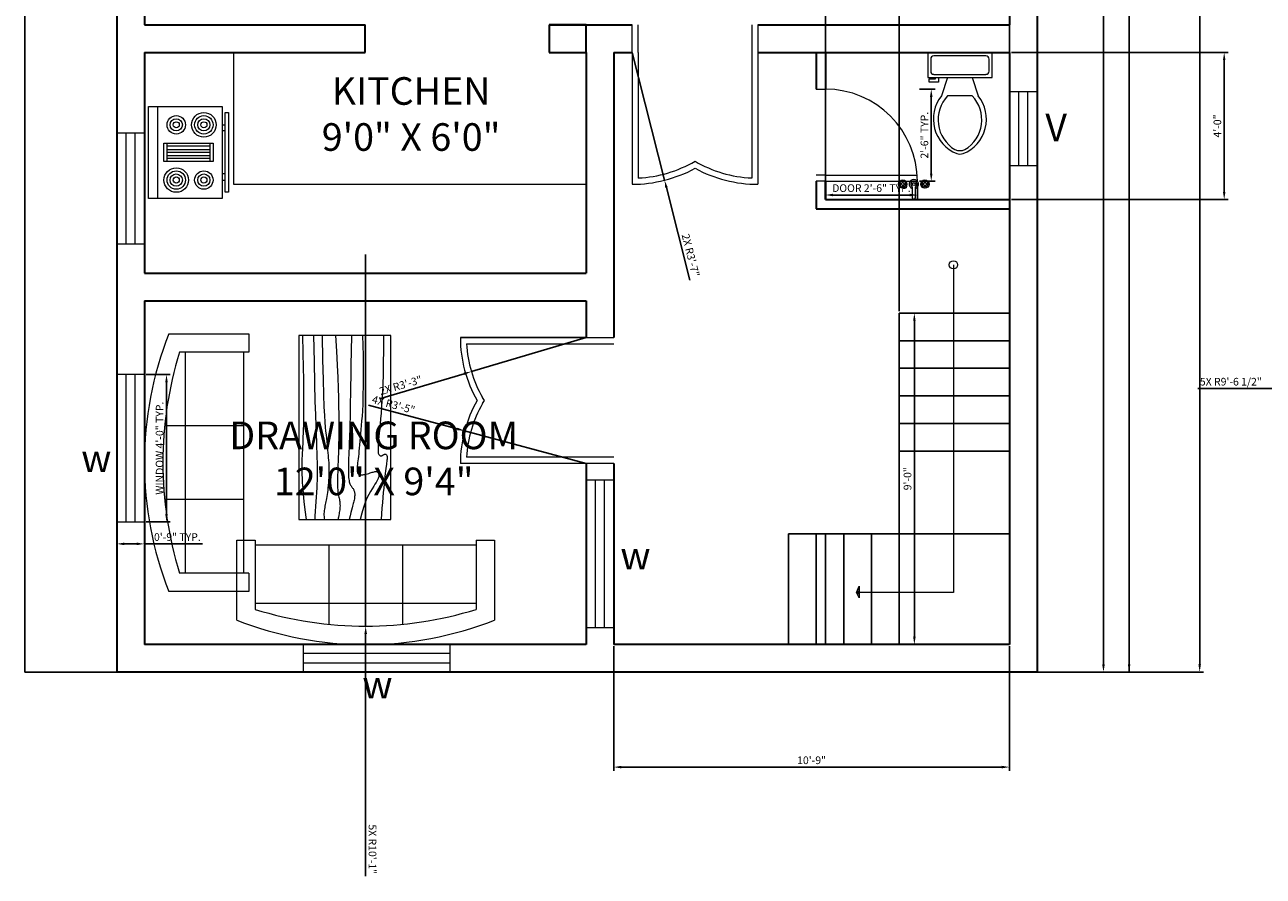
# Model space of a CAD drawing. Units: inches. Extents: x 2009 to 2890, y 2827 to 3504.
# Tile 1 of 6: x 2046 to 2449, y 2827 to 3105. Entities that reach past the tile are written whole.
import ezdxf

# ---------------------------------------------------------------- set-up
doc = ezdxf.new("R2010")
doc.units = ezdxf.units.IN
for name, color, linetype, lineweight in [('A-ANNO-DIMS', 2, 'Continuous', 18), ('A-ANNO-SYMB', 2, 'Continuous', 18), ('A-ANNO-TEXT', 3, 'Continuous', 18), ('A-AREA-IDEN', 7, 'Continuous', 25), ('A-DOOR', 3, 'Continuous', 18), ('A-EQPM', 9, 'Continuous', 18), ('A-FLOR-CASE', 32, 'Continuous', 20), ('A-FLOR-FIXT', 9, 'Continuous', 18), ('A-FLOR-STRS', 7, 'Continuous', 25), ('A-FURN', 8, 'Continuous', 18), ('A-GLAZ', 4, 'Continuous', 18), ('A-WALL', 7, 'Continuous', 35), ('C-PROP', 8, 'Continuous', 25)]:
    doc.layers.add(name, color=color, linetype=linetype, lineweight=lineweight)
doc.styles.get("Standard").update_dxf_attribs({"font": 'arial.ttf'})
doc.dimstyles.new('ISO-25', dxfattribs={"dimtxt": 2.5, "dimasz": 2.5, "dimexe": 1.25, "dimexo": 0.625, "dimtad": 1, "dimdec": 0, "dimlunit": 3, "dimtxsty": 'Standard', "dimcen": 2.5, "dimadec": 0, "dimazin": 0, "dimtfac": 1, "dimtdec": 0, "dimtmove": 0, "dimatfit": 3, "dimfxl": 1, "dimarcsym": 0})

# ---------------------------------------------------------------- blocks, each defined once
blk = doc.blocks.new('Table - Rectangular Woodgrain 60 x 30 in.')
for p, q in [((0, 0), (0, -30)), ((60, 0), (0, 0)), ((60, -30), (60, 0)), ((0, -30), (60, -30))]:
    blk.add_line(p, q)
for points in [[(0, -2.4), (4.8155, -2.418), (9.0302, -2.4688), (12.709, -2.5477), (15.9167, -2.65), (18.7181, -2.7711), (21.1781, -2.9063), (23.3616, -3.0508), (25.3333, -3.2), (27.1477, -3.3495), (28.8172, -3.4958), (30.3437, -3.636), (31.7291, -3.7667), (32.9756, -3.8849), (34.0849, -3.9875), (35.059, -4.0714), (35.9, -4.1334), (36.6114, -4.1711), (37.2041, -4.1854), (37.6906, -4.1779), (38.0833, -4.15), (38.3948, -4.1034), (38.6375, -4.0396), (38.8239, -3.9602), (38.9666, -3.8667), (39.0764, -3.7608), (39.1573, -3.6448), (39.2116, -3.521), (39.2416, -3.3917), (39.2498, -3.2593), (39.2385, -3.1261), (39.21, -2.9944), (39.1666, -2.8667), (39.111, -2.7447), (39.0468, -2.6281), (38.978, -2.5163), (38.9083, -2.4083), (38.8418, -2.3035), (38.7823, -2.201), (38.7337, -2.1001), (38.7, -2), (38.6844, -1.9003), (38.6875, -1.8021), (38.7094, -1.707), (38.75, -1.6167), (38.8094, -1.5326), (38.8875, -1.4563), (38.9844, -1.3893), (39.1, -1.3333), (39.2351, -1.2896), (39.3937, -1.2583), (39.5804, -1.2396), (39.8, -1.2333), (40.057, -1.2396), (40.3562, -1.2583), (40.7023, -1.2896), (41.1, -1.3333), (41.5547, -1.3895), (42.0755, -1.4573), (42.6721, -1.5361), (43.3542, -1.625), (44.1316, -1.7233), (45.014, -1.8302), (46.0114, -1.9449), (47.1333, -2.0667), (48.3862, -2.1947), (49.7625, -2.3281), (51.2513, -2.4663), (52.8416, -2.6083), (54.5226, -2.7535), (56.2833, -2.9011), (58.1127, -3.0501), (60, -3.2)], [(0, -9.2), (6.5759, -9.0858), (11.9385, -9.0365), (16.2527, -9.0418), (19.6833, -9.0917), (22.3952, -9.1759), (24.5531, -9.2844), (26.322, -9.4069), (27.8666, -9.5333), (29.3241, -9.6553), (30.7203, -9.7719), (32.0532, -9.8837), (33.3208, -9.9917), (34.5213, -10.0965), (35.6526, -10.199), (36.7128, -10.2999), (37.7, -10.4), (38.6129, -10.4996), (39.4531, -10.5969), (40.223, -10.6895), (40.925, -10.775), (41.5613, -10.8512), (42.1344, -10.9156), (42.6465, -10.966), (43.1, -11), (43.4976, -11.0158), (43.8437, -11.0136), (44.143, -10.9942), (44.4, -10.9583), (44.6195, -10.9069), (44.8062, -10.8406), (44.9648, -10.7603), (45.1, -10.6667), (45.2155, -10.5598), (45.3114, -10.4365), (45.3871, -10.2929), (45.4416, -10.125), (45.4743, -9.929), (45.4844, -9.7011), (45.4709, -9.4371), (45.4333, -9.1333), (45.3716, -8.7883), (45.2896, -8.4104), (45.1919, -8.0107), (45.0833, -7.6), (44.9685, -7.1893), (44.8521, -6.7896), (44.7388, -6.4117), (44.6333, -6.0667), (44.54, -5.7628), (44.4614, -5.4979), (44.4001, -5.2675), (44.3583, -5.0667), (44.3384, -4.8909), (44.3427, -4.7354), (44.3736, -4.5956), (44.4333, -4.4667), (44.5236, -4.3453), (44.6427, -4.2333), (44.7884, -4.1339), (44.9583, -4.05), (45.1501, -3.9849), (45.3614, -3.9417), (45.59, -3.9234), (45.8333, -3.9333), (46.0915, -3.9749), (46.3734, -4.0531), (46.6906, -4.1736), (47.0542, -4.3417), (47.4756, -4.5629), (47.9661, -4.8427), (48.5372, -5.1866), (49.2, -5.6), (49.9676, -6.0844), (50.8594, -6.625), (51.8965, -7.2031), (53.1, -7.8), (54.491, -8.3969), (56.0906, -8.975), (57.9199, -9.5156), (60, -10)], [(0, -12.8), (5.1847, -12.9322), (9.6213, -13.0323), (13.3963, -13.1059), (16.5958, -13.1583), (19.3063, -13.1952), (21.614, -13.2219), (23.6054, -13.2439), (25.3666, -13.2667), (26.9728, -13.2947), (28.4531, -13.3281), (29.8256, -13.3663), (31.1083, -13.4083), (32.3191, -13.4535), (33.476, -13.501), (34.597, -13.5501), (35.7, -13.6), (36.7984, -13.6497), (37.8875, -13.6979), (38.9578, -13.743), (40, -13.7833), (41.0047, -13.8174), (41.9625, -13.8438), (42.864, -13.8607), (43.7, -13.8667), (44.4631, -13.8604), (45.1552, -13.8417), (45.7801, -13.8104), (46.3416, -13.7667), (46.8439, -13.7104), (47.2906, -13.6417), (47.6858, -13.5604), (48.0333, -13.4667), (48.3375, -13.3608), (48.6042, -13.2448), (48.8396, -13.121), (49.05, -12.9917), (49.2417, -12.8593), (49.4208, -12.7261), (49.5937, -12.5944), (49.7667, -12.4667), (49.9452, -12.3451), (50.1323, -12.2313), (50.3303, -12.1268), (50.5416, -12.0333), (50.7686, -11.9524), (51.0135, -11.8854), (51.2788, -11.8341), (51.5666, -11.8), (51.8785, -11.7843), (52.2116, -11.7865), (52.562, -11.8059), (52.926, -11.8417), (53.2998, -11.8931), (53.6795, -11.9594), (54.0614, -12.0397), (54.4416, -12.1333), (54.8223, -12.2401), (55.2293, -12.3625), (55.6942, -12.5037), (56.2489, -12.6667), (56.9251, -12.8547), (57.7545, -13.0708), (58.7689, -13.3182), (60, -13.6)], [(0, -18), (5.124, -17.7273), (9.6609, -17.5057), (13.6705, -17.3303), (17.2125, -17.1958), (20.3467, -17.0973), (23.1328, -17.0297), (25.6307, -16.9878), (27.9, -16.9667), (29.9928, -16.9617), (31.9302, -16.9703), (33.7254, -16.9907), (35.3917, -17.0208), (36.9423, -17.0588), (38.3906, -17.1026), (39.7499, -17.1503), (41.0333, -17.2), (42.2519, -17.2496), (43.4073, -17.2969), (44.4986, -17.3395), (45.525, -17.375), (46.4858, -17.4012), (47.3802, -17.4156), (48.2074, -17.416), (48.9667, -17.4), (49.6583, -17.3662), (50.2872, -17.3167), (50.8595, -17.2547), (51.3812, -17.1833), (51.8584, -17.1057), (52.2971, -17.025), (52.7034, -16.9443), (53.0833, -16.8667), (53.443, -16.7951), (53.789, -16.7313), (54.128, -16.6768), (54.4666, -16.6334), (54.8115, -16.6024), (55.1693, -16.5854), (55.5465, -16.5841), (55.95, -16.6), (56.3828, -16.6337), (56.8346, -16.6823), (57.2915, -16.7418), (57.7396, -16.8084), (58.165, -16.878), (58.5539, -16.9469), (58.8924, -17.0111), (59.1666, -17.0667), (59.3679, -17.1107), (59.5078, -17.1438), (59.6032, -17.1675), (59.6708, -17.1833), (59.7275, -17.193), (59.7901, -17.1979), (59.8753, -17.1998), (60, -17.2)], [(0, -22.4), (8.0098, -22.2501), (14.4094, -22.1011), (19.4168, -21.9535), (23.25, -21.8083), (26.1269, -21.6663), (28.2656, -21.5281), (29.884, -21.3947), (31.2, -21.2667), (32.3967, -21.1448), (33.5172, -21.0292), (34.5697, -20.9198), (35.5625, -20.8167), (36.5037, -20.7198), (37.4015, -20.6292), (38.2642, -20.5448), (39.1, -20.4667), (39.9164, -20.3951), (40.7187, -20.3313), (41.5117, -20.2768), (42.3, -20.2333), (43.0883, -20.2024), (43.8812, -20.1854), (44.6836, -20.1841), (45.5, -20.2), (46.3328, -20.234), (47.1747, -20.2844), (48.0163, -20.3488), (48.8479, -20.425), (49.66, -20.5106), (50.4429, -20.6031), (51.1872, -20.7004), (51.8833, -20.8), (52.5246, -20.8999), (53.1166, -20.9995), (53.6681, -21.0983), (54.1875, -21.1958), (54.6834, -21.2919), (55.1646, -21.3859), (55.6394, -21.4777), (56.1167, -21.5667), (56.6028, -21.6515), (57.0961, -21.7266), (57.5929, -21.7852), (58.0896, -21.8208), (58.5823, -21.8268), (59.0674, -21.7964), (59.5412, -21.723), (60, -21.6)], [(0, -25.2), (8.6355, -25.0504), (15.7026, -24.9031), (21.4049, -24.7606), (25.9458, -24.625), (29.529, -24.4988), (32.3578, -24.3844), (34.6359, -24.284), (36.5667, -24.2), (38.3213, -24.1341), (39.9417, -24.0854), (41.437, -24.0523), (42.8167, -24.0333), (44.0901, -24.0268), (45.2667, -24.0313), (46.3557, -24.0451), (47.3667, -24.0667), (48.309, -24.0947), (49.1928, -24.1287), (50.0284, -24.168), (50.826, -24.2125), (51.5959, -24.2617), (52.3483, -24.3151), (53.0935, -24.3725), (53.8417, -24.4334), (54.6009, -24.497), (55.3699, -24.561), (56.1454, -24.6226), (56.9239, -24.6792), (57.7021, -24.7279), (58.4764, -24.7662), (59.2435, -24.7911), (60, -24.8)], [(0, -28.8), (5.6867, -28.6681), (10.45, -28.5698), (14.407, -28.5012), (17.675, -28.4584), (20.3711, -28.4374), (22.6125, -28.4344), (24.5164, -28.4455), (26.2, -28.4667), (27.762, -28.4947), (29.2276, -28.5281), (30.6033, -28.5663), (31.8958, -28.6084), (33.1118, -28.6535), (34.2578, -28.7011), (35.3405, -28.7501), (36.3666, -28.8), (37.3443, -28.8497), (38.288, -28.8974), (39.2137, -28.9412), (40.1375, -28.9792), (41.0753, -29.0093), (42.0432, -29.0297), (43.0572, -29.0384), (44.1333, -29.0333), (45.2936, -29.0114), (46.5843, -28.9641), (48.0579, -28.8816), (49.7666, -28.7542), (51.7629, -28.5721), (54.0989, -28.3255), (56.8272, -28.0048), (60, -27.6)]]:
    blk.add_lwpolyline(points)
blk = doc.blocks.new('Sofa - Roundback 7 ft.')
for p, q in [((-12.00002, -32.4421), (-12.00003, -6.5971)), ((11.99997, -32.4421), (11.99998, -6.5971)), ((-36.000027, -34), (-36.000027, -11.4696)), ((35.99998, -34), (35.99998, -11.4696)), ((-35.999844, -13.3819), (35.9998, -13.3819)), ((-36.000027, -32.4421), (35.99998, -32.4421))]:
    blk.add_line(p, q)
for points in [[(-36.000027, -34), (-42.000027, -34), (-42.000027, -8)], [(41.99998, -8), (41.99998, -34), (35.99998, -34)]]:
    blk.add_lwpolyline(points)
for centre, radius, start, end in [((0, -114.25), 114.25, 68.43141, 111.5686), ((-0.00001, -127.1968), 121.1968, 72.72033, 107.2797)]:
    blk.add_arc(centre, radius, start, end)
blk = doc.blocks.new('Range-Oven - 30 in top')
for p, q in [((0, -3), (30, -3)), ((12, -6), (18, -6)), ((13, -20), (13, -6)), ((14, -6), (14, -20)), ((15, -20), (15, -6)), ((16, -6), (16, -20)), ((17, -20), (17, -6)), ((18, -20), (12, -20)), ((6, -24), (6, -25)), ((8, -25), (8, -24)), ((22, -25), (22, -24)), ((24, -24), (24, -25))]:
    blk.add_line(p, q)
for points in [[(0, -24), (0, 0), (30, 0), (30, -24)], [(12, -21), (12, -5), (18, -5), (18, -21)], [(2, -26), (2, -25), (28, -25), (28, -26)]]:
    blk.add_lwpolyline(points, close=True)
for centre, radius in [((6, -9), 4), ((6, -9), 3), ((6, -9), 2), ((6, -9), 1), ((24, -9), 3), ((24, -9), 2), ((24, -9), 1), ((6, -18), 3), ((6, -18), 2), ((24, -18), 4), ((24, -18), 3), ((24, -18), 2), ((6, -18), 1), ((24, -18), 1)]:
    blk.add_circle(centre, radius)
blk = doc.blocks.new('Toilet - top')
for p, q in [((9.5, -6), (9.5, -2)), ((-8, -8.5), (-8, -8)), ((-7, -8), (-7, -9.5)), ((-4, -8), (-6, -14)), ((4, -8), (6, -14)), ((-10, -8.5), (-8, -8.5)), ((-10, -9.5), (-10, -8.5)), ((-7, -9.5), (-10, -9.5)), ((4, -14), (-4, -14))]:
    blk.add_line(p, q)
blk.add_lwpolyline([(10.5, -8), (10.5, 0), (-10.5, 0), (-10.5, -8)], close=True)
for points in [[(-9.5, -2), (-9.5, -6)], [(8.5, -1), (-8.5, -1)], [(-8.5, -7), (8.5, -7)]]:
    blk.add_lwpolyline(points)
for centre, radius, start, end in [((-8.62, -1.88), 0.884, 81.8699, 188.1301), ((8.62, -1.88), 0.884, 351.8699, 98.1301), ((-8.62, -6.12), 0.884, 171.8699, 278.1301), ((8.62, -6.12), 0.884, 261.8699, 8.1301), ((3.52, -21.58), 12.17, 141.4691, 247.9714), ((4.2, -21.82), 11.33, 136.3677, 238.9468), ((-3.52, -21.58), 12.17, 292.0284, 38.5307), ((-4.2, -21.82), 11.33, 301.053, 43.6321), ((0, -27.88), 4, 245.7318, 294.2682), ((0, -29), 4, 254.8605, 285.1395)]:
    blk.add_arc(centre, radius, start, end)
blk = doc.blocks.new('*D9')
at = {"layer": 'A-ANNO-DIMS', "color": 0, "lineweight": -2, "transparency": 16777216}
for p, q in [((2376.39, 3433.54), (2398.66, 3433.54)), ((2397.41, 3431.04), (2397.41, 2896.04)), ((2376.39, 2893.54), (2398.66, 2893.54))]:
    blk.add_line(p, q, dxfattribs=at)
at = {"layer": 'A-ANNO-DIMS', "color": 0, "transparency": 16777216}
for points in [[(2396.99, 3431.04), (2397.83, 3431.04), (2397.41, 3433.54)], [(2396.99, 2896.04), (2397.83, 2896.04), (2397.41, 2893.54)]]:
    blk.add_solid(points, dxfattribs=at)
at = {"layer": 'Defpoints', "color": 0, "transparency": 16777216}
for p in [(2375.76, 3433.54), (2375.76, 2893.54), (2397.41, 2893.54)]:
    blk.add_point(p, dxfattribs=at)
at = {"layer": 'A-ANNO-DIMS', "color": 0, "transparency": 16777216, "insert": (2395.51, 3163.54), "char_height": 2.5, "attachment_point": 5, "rotation": 90}
blk.add_mtext("45'", dxfattribs=at)
blk = doc.blocks.new('*D11')
at = {"layer": 'A-ANNO-DIMS', "color": 0, "lineweight": -2, "transparency": 16777216}
for p, q in [((2406.39, 3469.54), (2430.02, 3469.54)), ((2428.77, 3467.04), (2428.77, 2896.04)), ((2406.39, 2893.54), (2430.02, 2893.54))]:
    blk.add_line(p, q, dxfattribs=at)
at = {"layer": 'A-ANNO-DIMS', "color": 0, "transparency": 16777216}
for points in [[(2428.36, 3467.04), (2429.19, 3467.04), (2428.77, 3469.54)], [(2428.36, 2896.04), (2429.19, 2896.04), (2428.77, 2893.54)]]:
    blk.add_solid(points, dxfattribs=at)
at = {"layer": 'Defpoints', "color": 0, "transparency": 16777216}
for p in [(2405.76, 3469.54), (2405.76, 2893.54), (2428.77, 2893.54)]:
    blk.add_point(p, dxfattribs=at)
at = {"layer": 'A-ANNO-DIMS', "color": 0, "transparency": 16777216, "insert": (2426.87, 3181.54), "char_height": 2.5, "attachment_point": 5, "rotation": 90}
blk.add_mtext("48'", dxfattribs=at)
blk = doc.blocks.new('Faucet - Bathroom top')
for p, q in [((-4.107, 0.125), (-4.375, 0.125)), ((-3.75, 0.4788), (-3.75, 0.75)), ((-3.5, 0.482), (-3.5, 0.75)), ((-3.1461, 0.125), (-2.875, 0.125)), ((3.143, 0.125), (2.875, 0.125)), ((3.5, 0.4788), (3.5, 0.75)), ((3.75, 0.482), (3.75, 0.75)), ((4.1039, 0.125), (4.375, 0.125)), ((-4.1039, -0.125), (-4.375, -0.125)), ((-3.75, -0.4821), (-3.75, -0.75)), ((-3.5, -0.4789), (-3.5, -0.75)), ((-3.143, -0.125), (-2.875, -0.125)), ((-0.5, -0.8639), (-0.5, -4.5)), ((0.5, -4.5), (0.5, -0.8631)), ((3.1461, -0.125), (2.875, -0.125)), ((3.5, -0.4821), (3.5, -0.75)), ((3.75, -0.4789), (3.75, -0.75)), ((4.107, -0.125), (4.375, -0.125))]:
    blk.add_line(p, q)
for centre, radius in [((-3.625, 0), 1.375), ((-4.625, 0), 0.2795), ((-3.625, 0), 0.5), ((-3.625, 1), 0.2795), ((-2.625, 0), 0.2795), ((0, 0), 0.5), ((3.625, 0), 1.375), ((2.625, 0), 0.2795), ((3.625, 0), 0.5), ((3.625, 1), 0.2795), ((4.625, 0), 0.2795), ((-3.625, -1), 0.2795), ((3.625, -1), 0.2795)]:
    blk.add_circle(centre, radius)
for centre, radius, start, end in [((-3.625, 0), 1, 105.2407, 164.2093), ((-3.625, 0), 1, 16.44125, 74.07887), ((0, 0), 1.5, 289.6514, 250.3603), ((0, 0), 1, 300.3431, 239.7554), ((3.625, 0), 1, 106.12, 164.0884), ((3.625, 0), 1, 16.23422, 73.90469), ((-3.625, 0), 1, 196.2342, 253.9047), ((-3.625, 0), 1, 286.12, 344.0884), ((3.625, 0), 1, 196.4413, 254.0789), ((3.625, 0), 1, 285.2407, 344.2093), ((0, -4.5), 0.5, 180, 0)]:
    blk.add_arc(centre, radius, start, end)
blk = doc.blocks.new('*D18')
at = {"layer": 'A-ANNO-DIMS', "color": 0, "lineweight": -2, "transparency": 16777216}
for p, q in [((2376.39, 3433.54), (2407.01, 3433.54)), ((2405.76, 3431.04), (2405.76, 2896.04)), ((2376.39, 2893.54), (2407.01, 2893.54))]:
    blk.add_line(p, q, dxfattribs=at)
at = {"layer": 'A-ANNO-DIMS', "color": 0, "transparency": 16777216}
for points in [[(2405.35, 3431.04), (2406.18, 3431.04), (2405.76, 3433.54)], [(2405.35, 2896.04), (2406.18, 2896.04), (2405.76, 2893.54)]]:
    blk.add_solid(points, dxfattribs=at)
at = {"layer": 'Defpoints', "color": 0, "transparency": 16777216}
for p in [(2375.76, 3433.54), (2375.76, 2893.54), (2405.76, 2893.54)]:
    blk.add_point(p, dxfattribs=at)
at = {"layer": 'A-ANNO-DIMS', "color": 0, "transparency": 16777216, "insert": (2403.87, 3163.54), "char_height": 2.5, "attachment_point": 5, "rotation": 90}
blk.add_mtext("45'", dxfattribs=at)
blk = doc.blocks.new('*D19')
at = {"layer": 'A-ANNO-DIMS', "color": 0, "lineweight": -2, "transparency": 16777216}
for p, q in [((2376.39, 3433.54), (2407.01, 3433.54)), ((2405.76, 3431.04), (2405.76, 2896.04)), ((2376.39, 2893.54), (2407.01, 2893.54))]:
    blk.add_line(p, q, dxfattribs=at)
at = {"layer": 'A-ANNO-DIMS', "color": 0, "transparency": 16777216}
for points in [[(2405.35, 3431.04), (2406.18, 3431.04), (2405.76, 3433.54)], [(2405.35, 2896.04), (2406.18, 2896.04), (2405.76, 2893.54)]]:
    blk.add_solid(points, dxfattribs=at)
at = {"layer": 'Defpoints', "color": 0, "transparency": 16777216}
for p in [(2375.76, 3433.54), (2375.76, 2893.54), (2405.76, 2893.54)]:
    blk.add_point(p, dxfattribs=at)
at = {"layer": 'A-ANNO-DIMS', "color": 0, "transparency": 16777216, "insert": (2403.87, 3163.54), "char_height": 2.5, "attachment_point": 5, "rotation": 90}
blk.add_mtext("45'", dxfattribs=at)
blk = doc.blocks.new('WIN-48IN')
for p, q in [((0, 48), (0, 0)), ((9, 48), (0, 48)), ((3, 48), (3, 0)), ((6, 0), (6, 48)), ((9, 0), (9, 48)), ((0, 0), (9, 0))]:
    blk.add_line(p, q)
blk = doc.blocks.new('WIN-36IN')
for p, q in [((0, 36), (0, 0)), ((9, 36), (0, 36)), ((3, 36), (3, 0)), ((6, 0), (6, 36)), ((9, 0), (9, 36)), ((0, 0), (9, 0))]:
    blk.add_line(p, q)
blk = doc.blocks.new('VENT-24IN')
for p, q in [((0, 24), (0, 0)), ((9, 24), (0, 24)), ((3, 24), (3, 0)), ((6, 0), (6, 24)), ((9, 0), (9, 24)), ((0, 0), (9, 0))]:
    blk.add_line(p, q)
blk = doc.blocks.new('DOOR-30IN')
for p, q in [((0, 2), (30, 2)), ((0, 0), (30, 0))]:
    blk.add_line(p, q)
blk.add_arc((0, 0), 30, 0, 90)
blk = doc.blocks.new('*D31')
at = {"layer": 'A-ANNO-DIMS', "color": 0, "lineweight": -2, "transparency": 16777216}
for p, q in [((2085.39, 2990.51), (2093.21, 2990.51)), ((2091.96, 2945.01), (2091.96, 2988.01)), ((2085.39, 2942.51), (2093.21, 2942.51))]:
    blk.add_line(p, q, dxfattribs=at)
at = {"layer": 'A-ANNO-DIMS', "color": 0, "transparency": 16777216}
for points in [[(2091.55, 2988.01), (2092.38, 2988.01), (2091.96, 2990.51)], [(2091.55, 2945.01), (2092.38, 2945.01), (2091.96, 2942.51)]]:
    blk.add_solid(points, dxfattribs=at)
at = {"layer": 'Defpoints', "color": 0, "transparency": 16777216}
for p in [(2084.76, 2990.51), (2091.96, 2990.51), (2084.76, 2942.51)]:
    blk.add_point(p, dxfattribs=at)
at = {"layer": 'A-ANNO-DIMS', "color": 0, "transparency": 16777216, "insert": (2090.04, 2966.51), "char_height": 2.5, "attachment_point": 5, "rotation": 90}
blk.add_mtext('WINDOW 4\'-0" TYP.', dxfattribs=at)
blk = doc.blocks.new('*D32')
at = {"layer": 'A-ANNO-DIMS', "color": 0, "lineweight": -2, "transparency": 16777216}
for p, q in [((2075.76, 2941.88), (2075.76, 2934.06)), ((2084.76, 2941.88), (2084.76, 2934.06)), ((2078.26, 2935.31), (2082.26, 2935.31)), ((2084.76, 2935.31), (2103.75, 2935.31))]:
    blk.add_line(p, q, dxfattribs=at)
at = {"layer": 'A-ANNO-DIMS', "color": 0, "transparency": 16777216}
for points in [[(2078.26, 2935.73), (2078.26, 2934.89), (2075.76, 2935.31)], [(2082.26, 2935.73), (2082.26, 2934.89), (2084.76, 2935.31)]]:
    blk.add_solid(points, dxfattribs=at)
at = {"layer": 'Defpoints', "color": 0, "transparency": 16777216}
for p in [(2075.76, 2942.51), (2084.76, 2942.51), (2084.76, 2935.31)]:
    blk.add_point(p, dxfattribs=at)
at = {"layer": 'A-ANNO-DIMS', "color": 0, "transparency": 16777216, "insert": (2095.51, 2937.21), "char_height": 2.5, "attachment_point": 5}
blk.add_mtext('0\'-9" TYP.', dxfattribs=at)
blk = doc.blocks.new('*D41')
at = {"layer": 'A-ANNO-DIMS', "color": 0, "lineweight": -2, "transparency": 16777216}
for p, q in [((2306.76, 3052.91), (2306.76, 3047.79)), ((2336.76, 3052.91), (2336.76, 3047.79)), ((2309.26, 3049.04), (2334.26, 3049.04))]:
    blk.add_line(p, q, dxfattribs=at)
at = {"layer": 'A-ANNO-DIMS', "color": 0, "transparency": 16777216}
for points in [[(2309.26, 3049.46), (2309.26, 3048.62), (2306.76, 3049.04)], [(2334.26, 3049.46), (2334.26, 3048.62), (2336.76, 3049.04)]]:
    blk.add_solid(points, dxfattribs=at)
at = {"layer": 'Defpoints', "color": 0, "transparency": 16777216}
for p in [(2306.76, 3053.54), (2336.76, 3053.54), (2336.76, 3049.04)]:
    blk.add_point(p, dxfattribs=at)
at = {"layer": 'A-ANNO-DIMS', "color": 0, "transparency": 16777216, "insert": (2321.76, 3050.96), "char_height": 2.5, "attachment_point": 5}
blk.add_mtext('DOOR 2\'-6" TYP.', dxfattribs=at)
blk = doc.blocks.new('*D42')
at = {"layer": 'A-ANNO-DIMS', "color": 0, "lineweight": -2, "transparency": 16777216}
for p, q in [((2337.39, 3083.54), (2342.51, 3083.54)), ((2341.26, 3056.04), (2341.26, 3081.04)), ((2337.39, 3053.54), (2342.51, 3053.54))]:
    blk.add_line(p, q, dxfattribs=at)
at = {"layer": 'A-ANNO-DIMS', "color": 0, "transparency": 16777216}
for points in [[(2340.85, 3081.04), (2341.68, 3081.04), (2341.26, 3083.54)], [(2340.85, 3056.04), (2341.68, 3056.04), (2341.26, 3053.54)]]:
    blk.add_solid(points, dxfattribs=at)
at = {"layer": 'Defpoints', "color": 0, "transparency": 16777216}
for p in [(2336.76, 3083.54), (2341.26, 3083.54), (2336.76, 3053.54)]:
    blk.add_point(p, dxfattribs=at)
at = {"layer": 'A-ANNO-DIMS', "color": 0, "transparency": 16777216, "insert": (2339.36, 3068.54), "char_height": 2.5, "attachment_point": 5, "rotation": 90}
blk.add_mtext('2\'-6" TYP.', dxfattribs=at)
blk = doc.blocks.new('*D65')
at = {"layer": 'A-ANNO-DIMS', "color": 0, "lineweight": -2, "transparency": 16777216}
for p, q in [((2237.76, 2901.91), (2237.76, 2861.29)), ((2366.76, 2901.91), (2366.76, 2861.29)), ((2240.26, 2862.54), (2364.26, 2862.54))]:
    blk.add_line(p, q, dxfattribs=at)
at = {"layer": 'A-ANNO-DIMS', "color": 0, "transparency": 16777216}
for points in [[(2240.26, 2862.96), (2240.26, 2862.12), (2237.76, 2862.54)], [(2364.26, 2862.96), (2364.26, 2862.12), (2366.76, 2862.54)]]:
    blk.add_solid(points, dxfattribs=at)
at = {"layer": 'Defpoints', "color": 0, "transparency": 16777216}
for p in [(2237.76, 2902.54), (2366.76, 2902.54), (2366.76, 2862.54)]:
    blk.add_point(p, dxfattribs=at)
at = {"layer": 'A-ANNO-DIMS', "color": 0, "transparency": 16777216, "insert": (2302.26, 2864.44), "char_height": 2.5, "attachment_point": 5}
blk.add_mtext('10\'-9"', dxfattribs=at)
blk = doc.blocks.new('*D66')
at = {"layer": 'A-ANNO-DIMS', "color": 0, "lineweight": -2, "transparency": 16777216}
for p, q in [((2330.76, 3011.16), (2330.76, 3501.79)), ((2333.26, 3500.54), (2364.26, 3500.54)), ((2366.76, 3011.16), (2366.76, 3501.79))]:
    blk.add_line(p, q, dxfattribs=at)
at = {"layer": 'A-ANNO-DIMS', "color": 0, "transparency": 16777216}
for points in [[(2333.26, 3500.96), (2333.26, 3500.12), (2330.76, 3500.54)], [(2364.26, 3500.96), (2364.26, 3500.12), (2366.76, 3500.54)]]:
    blk.add_solid(points, dxfattribs=at)
at = {"layer": 'Defpoints', "color": 0, "transparency": 16777216}
for p in [(2366.76, 3500.54), (2330.76, 3010.54), (2366.76, 3010.54)]:
    blk.add_point(p, dxfattribs=at)
at = {"layer": 'A-ANNO-DIMS', "color": 0, "transparency": 16777216, "insert": (2348.76, 3502.44), "char_height": 2.5, "attachment_point": 5}
blk.add_mtext('3\'-0"', dxfattribs=at)
blk = doc.blocks.new('*D67')
at = {"layer": 'A-ANNO-DIMS', "color": 0, "lineweight": -2, "transparency": 16777216}
for p, q in [((2366.14, 3010.54), (2334.51, 3010.54)), ((2335.76, 2905.04), (2335.76, 3008.04)), ((2366.14, 2902.54), (2334.51, 2902.54))]:
    blk.add_line(p, q, dxfattribs=at)
at = {"layer": 'A-ANNO-DIMS', "color": 0, "transparency": 16777216}
for points in [[(2335.35, 3008.04), (2336.18, 3008.04), (2335.76, 3010.54)], [(2335.35, 2905.04), (2336.18, 2905.04), (2335.76, 2902.54)]]:
    blk.add_solid(points, dxfattribs=at)
at = {"layer": 'Defpoints', "color": 0, "transparency": 16777216}
for p in [(2335.76, 3010.54), (2366.76, 3010.54), (2366.76, 2902.54)]:
    blk.add_point(p, dxfattribs=at)
at = {"layer": 'A-ANNO-DIMS', "color": 0, "transparency": 16777216, "insert": (2333.86, 2956.54), "char_height": 2.5, "attachment_point": 5, "rotation": 90}
blk.add_mtext('9\'-0"', dxfattribs=at)
blk = doc.blocks.new('*D68')
at = {"layer": 'A-ANNO-DIMS', "color": 0, "lineweight": -2, "transparency": 16777216}
for p, q in [((2306.76, 3048.16), (2306.76, 3501.79)), ((2309.26, 3500.54), (2364.26, 3500.54)), ((2366.76, 3048.16), (2366.76, 3501.79))]:
    blk.add_line(p, q, dxfattribs=at)
at = {"layer": 'A-ANNO-DIMS', "color": 0, "transparency": 16777216}
for points in [[(2309.26, 3500.96), (2309.26, 3500.12), (2306.76, 3500.54)], [(2364.26, 3500.96), (2364.26, 3500.12), (2366.76, 3500.54)]]:
    blk.add_solid(points, dxfattribs=at)
at = {"layer": 'Defpoints', "color": 0, "transparency": 16777216}
for p in [(2366.76, 3500.54), (2306.76, 3047.54), (2366.76, 3047.54)]:
    blk.add_point(p, dxfattribs=at)
at = {"layer": 'A-ANNO-DIMS', "color": 0, "transparency": 16777216, "insert": (2336.76, 3502.44), "char_height": 2.5, "attachment_point": 5}
blk.add_mtext('5\'-0"', dxfattribs=at)
blk = doc.blocks.new('*D69')
at = {"layer": 'A-ANNO-DIMS', "color": 0, "lineweight": -2, "transparency": 16777216}
for p, q in [((2367.39, 3095.54), (2438.01, 3095.54)), ((2436.76, 3050.04), (2436.76, 3093.04)), ((2367.39, 3047.54), (2438.01, 3047.54))]:
    blk.add_line(p, q, dxfattribs=at)
at = {"layer": 'A-ANNO-DIMS', "color": 0, "transparency": 16777216}
for points in [[(2436.35, 3093.04), (2437.18, 3093.04), (2436.76, 3095.54)], [(2436.35, 3050.04), (2437.18, 3050.04), (2436.76, 3047.54)]]:
    blk.add_solid(points, dxfattribs=at)
at = {"layer": 'Defpoints', "color": 0, "transparency": 16777216}
for p in [(2366.76, 3095.54), (2436.76, 3095.54), (2366.76, 3047.54)]:
    blk.add_point(p, dxfattribs=at)
at = {"layer": 'A-ANNO-DIMS', "color": 0, "transparency": 16777216, "insert": (2434.86, 3071.54), "char_height": 2.5, "attachment_point": 5, "rotation": 90}
blk.add_mtext('4\'-0"', dxfattribs=at)
blk = doc.blocks.new('*D83')
at = {"layer": 'A-ANNO-DIMS', "color": 0, "lineweight": -2, "transparency": 16777216}
for p, q in [((2243.76, 3095.54), (2254.34, 3053.86)), ((2262.61, 3021.24), (2254.95, 3051.44))]:
    blk.add_line(p, q, dxfattribs=at)
at = {"layer": 'A-ANNO-DIMS', "color": 0, "transparency": 16777216}
blk.add_solid([(2255.36, 3051.54), (2254.55, 3051.33), (2254.34, 3053.86)], dxfattribs=at)
at = {"layer": 'Defpoints', "color": 0, "transparency": 16777216}
for p in [(2243.76, 3095.54), (2254.34, 3053.86)]:
    blk.add_point(p, dxfattribs=at)
at = {"layer": 'A-ANNO-DIMS', "color": 0, "transparency": 16777216, "insert": (2262.53, 3029.32), "char_height": 2.5, "attachment_point": 5, "rotation": 284.2368}
blk.add_mtext('2X R3\'-7"', dxfattribs=at)
blk = doc.blocks.new('*D84')
at = {"layer": 'A-ANNO-DIMS', "color": 0, "lineweight": -2, "transparency": 16777216}
for p, q in [((2157.79, 2980.56), (2186.74, 2972.8)), ((2228.76, 2961.54), (2189.16, 2972.15))]:
    blk.add_line(p, q, dxfattribs=at)
at = {"layer": 'A-ANNO-DIMS', "color": 0, "transparency": 16777216}
blk.add_solid([(2186.85, 2973.2), (2186.64, 2972.39), (2189.16, 2972.15)], dxfattribs=at)
at = {"layer": 'Defpoints', "color": 0, "transparency": 16777216}
for p in [(2189.16, 2972.15), (2228.76, 2961.54)]:
    blk.add_point(p, dxfattribs=at)
at = {"layer": 'A-ANNO-DIMS', "color": 0, "transparency": 16777216, "insert": (2165.89, 2980.35), "char_height": 2.5, "attachment_point": 5, "rotation": 345.0006}
blk.add_mtext('4X R3\'-5"', dxfattribs=at)
blk = doc.blocks.new('*D85')
at = {"layer": 'A-ANNO-DIMS', "color": 0, "lineweight": -2, "transparency": 16777216}
for p, q in [((2228.76, 3002.54), (2191.36, 2991.48)), ((2161.39, 2982.62), (2188.97, 2990.77))]:
    blk.add_line(p, q, dxfattribs=at)
at = {"layer": 'A-ANNO-DIMS', "color": 0, "transparency": 16777216}
blk.add_solid([(2188.85, 2991.17), (2189.08, 2990.37), (2191.36, 2991.48)], dxfattribs=at)
at = {"layer": 'Defpoints', "color": 0, "transparency": 16777216}
for p in [(2228.76, 3002.54), (2191.36, 2991.48)]:
    blk.add_point(p, dxfattribs=at)
at = {"layer": 'A-ANNO-DIMS', "color": 0, "transparency": 16777216, "insert": (2168.38, 2986.67), "char_height": 2.5, "attachment_point": 5, "rotation": 16.4698}
blk.add_mtext('2X R3\'-3"', dxfattribs=at)
blk = doc.blocks.new('*D86')
at = {"layer": 'A-ANNO-DIMS', "color": 0, "lineweight": -2, "transparency": 16777216}
for p, q in [((2156.89, 3029.68), (2156.89, 2908.48)), ((2156.89, 2826.96), (2156.89, 2905.98))]:
    blk.add_line(p, q, dxfattribs=at)
at = {"layer": 'A-ANNO-DIMS', "color": 0, "transparency": 16777216}
blk.add_solid([(2157.31, 2905.98), (2156.48, 2905.98), (2156.89, 2908.48)], dxfattribs=at)
at = {"layer": 'Defpoints', "color": 0, "transparency": 16777216}
for p in [(2156.89, 3029.68), (2156.89, 2908.48)]:
    blk.add_point(p, dxfattribs=at)
at = {"layer": 'A-ANNO-DIMS', "color": 0, "transparency": 16777216, "insert": (2158.79, 2835.76), "char_height": 2.5, "attachment_point": 5, "rotation": 270.0002}
blk.add_mtext('5X R10\'-1"', dxfattribs=at)
blk = doc.blocks.new('*D87')
at = {"layer": 'A-ANNO-DIMS', "color": 0, "lineweight": -2, "transparency": 16777216}
for p, q in [((2428.19, 2985.94), (2504.98, 2985.94)), ((2621.73, 2985.94), (2507.48, 2985.94))]:
    blk.add_line(p, q, dxfattribs=at)
at = {"layer": 'A-ANNO-DIMS', "color": 0, "transparency": 16777216}
blk.add_solid([(2504.98, 2986.36), (2504.98, 2985.53), (2507.48, 2985.94)], dxfattribs=at)
at = {"layer": 'Defpoints', "color": 0, "transparency": 16777216}
for p in [(2507.48, 2985.94), (2621.73, 2985.94)]:
    blk.add_point(p, dxfattribs=at)
at = {"layer": 'A-ANNO-DIMS', "color": 0, "transparency": 16777216, "insert": (2438.93, 2987.86), "char_height": 2.5, "attachment_point": 5, "rotation": 0.0001}
blk.add_mtext('5X R9\'-6 1/2"', dxfattribs=at)

msp = doc.modelspace()

# ---------------------------------------------------------------- linework, layer by layer
at = {"layer": 'A-ANNO-SYMB'}
for p, q in [((2348.5, 3026.27), (2348.5, 2919.51)), ((2316.91, 2919.5), (2317.75, 2921.5)), ((2316.91, 2919.5), (2317.75, 2920.09)), ((2317.75, 2919.51), (2316.91, 2919.5)), ((2317.75, 2917.73), (2316.91, 2919.5)), ((2317.75, 2918.85), (2316.91, 2919.5)), ((2317.75, 2919.51), (2317.75, 2921.5)), ((2317.75, 2921.5), (2317.75, 2917.73)), ((2317.75, 2921.5), (2317.75, 2919.51)), ((2317.75, 2920.09), (2317.75, 2919.51)), ((2348.5, 2919.51), (2317.75, 2919.51)), ((2317.75, 2919.51), (2317.75, 2918.85))]:
    msp.add_line(p, q, dxfattribs=at)
msp.add_circle((2348.5, 3026.27), 1.34, dxfattribs=at)
at = {"layer": 'A-DOOR'}
for p, q in [((2243.76, 3095.54), (2243.76, 3104.54)), ((2245.76, 3095.54), (2245.76, 3104.54)), ((2282.76, 3104.54), (2282.76, 3095.54)), ((2284.76, 3104.54), (2284.76, 3095.54)), ((2243.76, 3095.54), (2243.76, 3054.54)), ((2245.76, 3095.54), (2245.76, 3054.54)), ((2282.76, 3095.54), (2282.76, 3054.54)), ((2284.76, 3095.54), (2284.76, 3054.54)), ((2303.76, 3083.54), (2306.76, 3083.54)), ((2243.76, 3054.54), (2243.76, 3052.54)), ((2284.76, 3054.54), (2284.76, 3052.54)), ((2306.76, 3055.54), (2303.76, 3055.54)), ((2306.76, 3053.54), (2303.76, 3053.54)), ((2228.76, 3002.54), (2187.76, 3002.54)), ((2187.76, 3002.54), (2228.76, 3002.54)), ((2187.76, 3000.54), (2187.81, 3000.54)), ((2189.81, 3000.54), (2228.76, 3000.54)), ((2228.76, 3002.54), (2237.76, 3002.54)), ((2228.76, 3002.54), (2228.76, 3002.54)), ((2228.76, 3000.54), (2237.76, 3000.54)), ((2237.76, 3002.54), (2237.76, 3002.54)), ((2195.59, 2982.04), (2194.99, 2983.04)), ((2194.99, 2981.04), (2195.59, 2982.04)), ((2187.81, 2963.54), (2187.76, 2963.54)), ((2228.76, 2963.54), (2189.81, 2963.54)), ((2237.76, 2963.54), (2228.76, 2963.54)), ((2228.76, 2961.54), (2187.76, 2961.54)), ((2237.76, 2961.54), (2228.76, 2961.54))]:
    msp.add_line(p, q, dxfattribs=at)
for centre, radius, start, end in [((2243.76, 3095.54), 43, 270, 298.473), ((2243.76, 3095.54), 41, 272.796, 300), ((2284.76, 3095.54), 41, 240, 267.204), ((2284.76, 3095.54), 43, 241.527, 270), ((2228.76, 3002.54), 41, 180, 210), ((2228.76, 3002.54), 39, 182.9395, 210), ((2228.76, 2961.54), 41, 150, 180), ((2228.76, 2961.54), 39, 150, 177.0605)]:
    msp.add_arc(centre, radius, start, end, dxfattribs=at)
at = {"layer": 'A-FLOR-CASE'}
for p, q in [((2113.76, 3095.54), (2113.76, 3052.54)), ((2113.76, 3052.54), (2228.76, 3052.54))]:
    msp.add_line(p, q, dxfattribs=at)
at = {"layer": 'A-FLOR-STRS'}
for p, q in [((2330.76, 3010.54), (2330.76, 2902.54)), ((2366.76, 3010.54), (2330.76, 3010.54)), ((2366.76, 3010.54), (2330.76, 3010.54)), ((2366.76, 3001.54), (2330.76, 3001.54)), ((2366.76, 2992.54), (2330.76, 2992.54)), ((2366.76, 2983.54), (2330.76, 2983.54)), ((2366.76, 2974.54), (2330.76, 2974.54)), ((2366.76, 2965.54), (2330.76, 2965.54)), ((2366.76, 2938.54), (2294.76, 2938.54)), ((2294.76, 2938.54), (2294.76, 2902.54)), ((2303.76, 2938.54), (2303.76, 2902.54)), ((2303.76, 2938.54), (2303.76, 2902.54)), ((2306.76, 2938.54), (2306.76, 2902.54)), ((2312.76, 2938.54), (2312.76, 2902.54)), ((2321.76, 2938.54), (2321.76, 2902.54))]:
    msp.add_line(p, q, dxfattribs=at)
at = {"layer": 'A-WALL'}
for p, q in [((2075.76, 3433.54), (2075.76, 2893.54)), ((2375.76, 3433.54), (2375.76, 2893.54)), ((2084.76, 3232.54), (2084.76, 3104.54)), ((2366.76, 3232.54), (2366.76, 3104.54)), ((2084.76, 3104.54), (2156.76, 3104.54)), ((2156.76, 3095.54), (2156.76, 3104.54)), ((2228.76, 3104.54), (2216.76, 3104.54)), ((2216.76, 3104.54), (2216.76, 3095.54)), ((2216.76, 3104.54), (2243.76, 3104.54)), ((2228.76, 3095.54), (2228.76, 3104.54)), ((2284.76, 3104.54), (2366.76, 3104.54)), ((2084.76, 3095.54), (2156.76, 3095.54)), ((2084.76, 3095.54), (2084.76, 3023.54)), ((2216.76, 3095.54), (2228.76, 3095.54)), ((2228.76, 3095.54), (2228.76, 3023.54)), ((2237.76, 3095.54), (2237.76, 3002.54)), ((2237.76, 3095.54), (2243.76, 3095.54)), ((2237.76, 3095.54), (2243.76, 3095.54)), ((2284.76, 3095.54), (2366.76, 3095.54)), ((2303.76, 3095.54), (2303.76, 3083.54)), ((2306.76, 3095.54), (2306.76, 3083.54)), ((2366.76, 3095.54), (2366.76, 2902.54)), ((2303.76, 3053.54), (2303.76, 3044.54)), ((2306.76, 3047.54), (2306.76, 3053.54)), ((2306.76, 3053.54), (2306.76, 3047.54)), ((2303.76, 3044.54), (2366.76, 3044.54)), ((2306.76, 3047.54), (2366.76, 3047.54)), ((2084.76, 3023.54), (2228.76, 3023.54)), ((2084.76, 3014.54), (2228.76, 3014.54)), ((2084.76, 3014.54), (2084.76, 2902.54)), ((2228.76, 3014.54), (2228.76, 3002.54)), ((2228.76, 3014.54), (2228.76, 3002.54)), ((2228.76, 2961.54), (2228.76, 2902.54)), ((2237.76, 2961.54), (2237.76, 2960.54)), ((2237.76, 2961.54), (2237.76, 2902.54)), ((2228.76, 2902.54), (2084.76, 2902.54)), ((2366.76, 2902.54), (2237.76, 2902.54)), ((2375.76, 2893.54), (2075.76, 2893.54))]:
    msp.add_line(p, q, dxfattribs=at)
at = {"layer": 'C-PROP'}
for p, q in [((2045.76, 3433.54), (2045.76, 2893.54)), ((2405.76, 3433.54), (2405.76, 2893.54)), ((2045.76, 2893.54), (2075.76, 2893.54)), ((2405.76, 2893.54), (2375.76, 2893.54))]:
    msp.add_line(p, q, dxfattribs=at)

# ---------------------------------------------------------------- block references
at = {"layer": 'A-DOOR'}
msp.add_blockref('DOOR-30IN', (2306.76, 3053.54), dxfattribs=at)
at = {"layer": 'A-EQPM', "rotation": 90}
msp.add_blockref('Range-Oven - 30 in top', (2086.14, 3047.92), dxfattribs=at)
at = {"layer": 'A-FLOR-FIXT'}
for name, p in [('Toilet - top', (2350.61, 3095.38)), ('Faucet - Bathroom top', (2335.59, 3052.6))]:
    msp.add_blockref(name, p, dxfattribs=at)
at = {"layer": 'A-FURN'}
for name, p, rotation in [('Sofa - Roundback 7 ft.', (2084.76, 2961.8), 90), ('Table - Rectangular Woodgrain 60 x 30 in.', (2165.11, 3003.27), 270.0000000000006), ('Sofa - Roundback 7 ft.', (2156.89, 2902.48), 180)]:
    msp.add_blockref(name, p, dxfattribs=dict(at, rotation=rotation))
at = {"layer": 'A-GLAZ'}
for name, p in [('VENT-24IN', (2366.76, 3058.63)), ('WIN-36IN', (2075.76, 3033.17)), ('WIN-48IN', (2075.76, 2942.51)), ('WIN-48IN', (2228.76, 2908.04))]:
    msp.add_blockref(name, p, dxfattribs=at)
at = {"layer": 'A-GLAZ', "rotation": 270.0000000000027}
msp.add_blockref('WIN-48IN', (2136.47, 2902.54), dxfattribs=at)

# ---------------------------------------------------------------- texts
at = {"layer": 'A-ANNO-TEXT', "char_height": 9, "attachment_point": 1}
for s, width, insert in [('\\pxqc;V', 57.7621, (2353.09, 3075.59)), ('\\pxqc;w', 53.6341, (2042.27, 2967.74)), ('\\pxqc;w', 53.6341, (2218.02, 2935.98)), ('\\pxqc;w', 53.6341, (2133.91, 2893.91))]:
    msp.add_mtext_dynamic_manual_height_columns(s, width=width, gutter_width=12.5, heights=[0], dxfattribs=dict(at, insert=insert))
at = {"layer": 'A-AREA-IDEN', "char_height": 9, "attachment_point": 1}
for s, width, insert in [('\\pxqc;KITCHEN\\P9\'0" X 6\'0"', 97.3998, (2123.01, 3087.45)), ('\\pxqc;DRAWING ROOM\\P12\'0" X 9\'4"', 123.1458, (2097.94, 2975.18))]:
    msp.add_mtext_dynamic_manual_height_columns(s, width=width, gutter_width=12.5, heights=[0], dxfattribs=dict(at, insert=insert))

# ---------------------------------------------------------------- dimensions: what is measured, and where the dimension line sits
at = {"layer": 'A-ANNO-DIMS'}
for base, p1, p2, picture, middle in [((2366.76, 3500.54), (2306.76, 3047.54), (2366.76, 3047.54), '*D68', (2336.76, 3502.44)), ((2366.76, 3500.54), (2330.76, 3010.54), (2366.76, 3010.54), '*D66', (2348.76, 3502.44)), ((2366.76, 2862.54), (2237.76, 2902.54), (2366.76, 2902.54), '*D65', (2302.26, 2864.44))]:
    dim = msp.add_linear_dim(base=base, p1=p1, p2=p2, dimstyle='ISO-25', override={"dimdec": 1, "dimlfac": 1, "dimrnd": 0, "dimzin": 1, "dimdsep": 46, "dimlunit": 4, "dimfrac": 2}, dxfattribs=at)
    dim.commit()
    dim.dimension.update_dxf_attribs({"geometry": picture, "text_midpoint": middle})
for base, p1, p2, override, picture, middle in [((2428.77, 2893.54), (2405.76, 3469.54), (2405.76, 2893.54), {"dimclrd": 0, "dimclre": 0, "dimclrt": 0}, '*D11', (2426.87, 3181.54)), ((2397.41, 2893.54), (2375.76, 3433.54), (2375.76, 2893.54), {"dimclrd": 0, "dimclre": 0, "dimclrt": 0}, '*D9', (2395.51, 3163.54)), ((2405.76, 2893.54), (2375.76, 3433.54), (2375.76, 2893.54), {"dimclrd": 0, "dimclre": 0, "dimclrt": 0}, '*D18', (2403.87, 3163.54)), ((2405.76, 2893.54), (2375.76, 3433.54), (2375.76, 2893.54), {"dimclrd": 0, "dimclre": 0, "dimclrt": 0}, '*D19', (2403.87, 3163.54)), ((2436.76, 3095.54), (2366.76, 3047.54), (2366.76, 3095.54), {"dimdec": 1, "dimlfac": 1, "dimrnd": 0, "dimzin": 1, "dimdsep": 46, "dimlunit": 4, "dimfrac": 2}, '*D69', (2434.86, 3071.54)), ((2335.76, 3010.54), (2366.76, 2902.54), (2366.76, 3010.54), {"dimdec": 1, "dimlfac": 1, "dimrnd": 0, "dimzin": 1, "dimdsep": 46, "dimlunit": 4, "dimfrac": 2}, '*D67', (2333.86, 2956.54))]:
    dim = msp.add_linear_dim(base=base, p1=p1, p2=p2, angle=90, dimstyle='ISO-25', override=override, dxfattribs=at)
    dim.commit()
    dim.dimension.update_dxf_attribs({"geometry": picture, "text_midpoint": middle})
for center, mpoint, text, picture, middle in [((2243.76, 3095.54), (2254.34, 3053.86), '2X <>', '*D83', (2260.68, 3028.85)), ((2156.89, 3029.68), (2156.89, 2908.48), '5X <>', '*D86', (2156.89, 2835.76)), ((2228.76, 3002.54), (2191.36, 2991.48), '2X <>', '*D85', (2168.92, 2984.85)), ((2621.732653, 2985.944293), (2507.482653, 2985.944), '5X <>', '*D87', (2438.932653, 2985.9438242)), ((2228.76, 2961.54), (2189.16, 2972.15), '4X <>', '*D84', (2165.4, 2978.52))]:
    dim = msp.add_radius_dim(center=center, mpoint=mpoint, text=text, dimstyle='ISO-25', override={"dimdec": 1, "dimlfac": 1, "dimrnd": 0, "dimzin": 1, "dimdsep": 46, "dimlunit": 4, "dimfrac": 2}, dxfattribs=at)
    dim.commit()
    dim.dimension.update_dxf_attribs({"geometry": picture, "text_midpoint": middle, "dimtype": 164})
for base, p1, p2, text, picture, middle in [((2341.26, 3083.54), (2336.76, 3053.54), (2336.76, 3083.54), '<> TYP.', '*D42', (2339.36, 3068.54)), ((2091.96, 2990.51), (2084.76, 2942.51), (2084.76, 2990.51), 'WINDOW <> TYP.', '*D31', (2090.04, 2966.51))]:
    dim = msp.add_linear_dim(base=base, p1=p1, p2=p2, angle=90, text=text, dimstyle='ISO-25', override={"dimdec": 1, "dimlfac": 1, "dimrnd": 0, "dimzin": 1, "dimdsep": 46, "dimlunit": 4, "dimfrac": 2}, dxfattribs=at)
    dim.commit()
    dim.dimension.update_dxf_attribs({"geometry": picture, "text_midpoint": middle})
for base, p1, p2, text, picture, middle in [((2336.76, 3049.04), (2306.76, 3053.54), (2336.76, 3053.54), 'DOOR <> TYP.', '*D41', (2321.76, 3050.96)), ((2084.76, 2935.31), (2075.76, 2942.51), (2084.76, 2942.51), '<> TYP.', '*D32', (2095.51, 2937.21))]:
    dim = msp.add_linear_dim(base=base, p1=p1, p2=p2, text=text, dimstyle='ISO-25', override={"dimdec": 1, "dimlfac": 1, "dimrnd": 0, "dimzin": 1, "dimdsep": 46, "dimlunit": 4, "dimfrac": 2}, dxfattribs=at)
    dim.commit()
    dim.dimension.update_dxf_attribs({"geometry": picture, "text_midpoint": middle})

doc.saveas('drawing.dxf')
